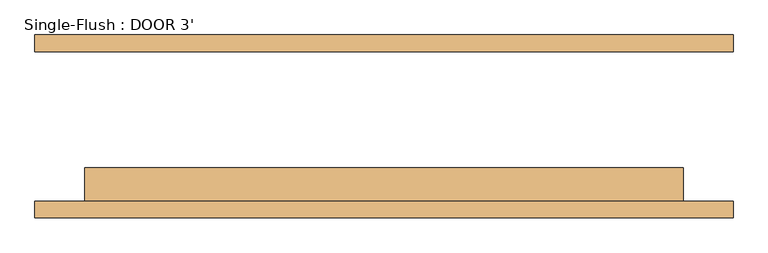
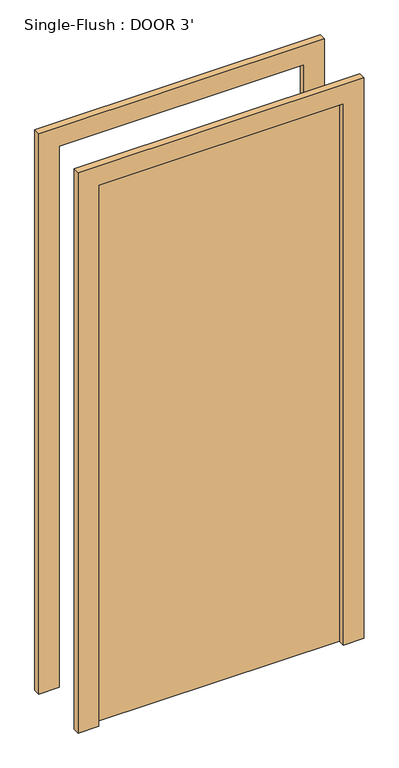
"""IFC4 building model written with IfcOpenShell, lengths in millimetres: door geometry, Single-Flush : DOOR 3'."""

from ifc_helpers import new_model, si_unit, frame, origin, origin_with_axes, place, context, project, spatial, polyline, outline, extrude, source, transform, mapped, element, save


def single_flush_door_3_a90ba1ad(model_context):
    return source(origin(), model_context, "Body", "SweptSolid", [
        extrude(outline(polyline([(2209.8, -533.4), (0.0, -533.4), (0.0, -457.2), (2133.6, -457.2), (2133.6, 457.2), (0.0, 457.2), (0.0, 533.4), (2209.8, 533.4), (2209.8, -533.4)])), frame((0.0, -139.7, 0.0), z_axis=(0.0, 1.0, 0.0), x_axis=(0.0, 0.0, 1.0)), (0.0, 0.0, 1.0), 25.4),
        extrude(outline(polyline([(2209.8, 533.4), (2209.8, -533.4), (0.0, -533.4), (0.0, -457.2), (2133.6, -457.2), (2133.6, 457.2), (0.0, 457.2), (0.0, 533.4), (2209.8, 533.4)])), frame((0.0, 114.3, 0.0), z_axis=(0.0, 1.0, 0.0), x_axis=(0.0, 0.0, 1.0)), (0.0, 0.0, 1.0), 25.4),
        extrude(outline(polyline([(457.2, -63.5), (457.2, -114.3), (-457.2, -114.3), (-457.2, -63.5), (457.2, -63.5)])), origin_with_axes(), (0.0, 0.0, 1.0), 2133.6),
    ])


if __name__ == "__main__":
    model = new_model("IFC4")
    model_context = context("Model", 3, world=origin())
    ifc_project = project(units=[si_unit("LENGTHUNIT", "METRE", prefix="MILLI")], contexts=[model_context])
    site = spatial("IfcSite", under=ifc_project)
    building = spatial("IfcBuilding", under=site)
    placement = place(None, origin())
    single_flush_door_3_shape = single_flush_door_3_a90ba1ad(model_context)
    element("IfcDoor", 1, ObjectType="Single-Flush : DOOR 3'", at=placement, inside=building, context=model_context, shape_type="MappedRepresentation", body=[
        mapped(single_flush_door_3_shape, transform((0.0, 0.0, 0.0), x_axis=(1.0, 0.0, 0.0), y_axis=(0.0, 1.0, 0.0), z_axis=(0.0, 0.0, 1.0))),
    ])
    save(model, "model.ifc")

# Revit data of these elements
# Type "Single-Flush : DOOR 3'"
#   Type Mark = "8"
#   Construction Type Id = "MDOOR"
#   Assembly Code = "C1020"
#   Analytic Construction = "Metal"
#   Thickness = 0' - 2"
#   Heat Transfer Coefficient (U) = 0.651978 BTU/(h·ft²·°F)
#   Height = 7' - 0"
#   Trim Projection Ext = 0' - 1"
#   Trim Projection Int = 0' - 1"
#   Trim Width = 0' - 3"
#   Width = 3' - 0"
#   Define Thermal Properties by = 1
#   Door Material = Door - Panel
#   Frame Material = Door - Frame
#   Visual Light Transmittance = 0
#   Solar Heat Gain Coefficient = 0
#   Function = (empty or 0)
#   Wall Closure = (empty or 0)
# Element 1 (IfcDoor, "Single-Flush : DOOR 3'")
#   Materials on its faces: "Door - Frame", "Door - Panel"
# Materials
#   "Door - Panel": class "Wood", colour RGB 210 159 95, transparency 0, Cost = 0
#   "Door - Frame": colour RGB 118 70 51, transparency 0, Cost = 0
